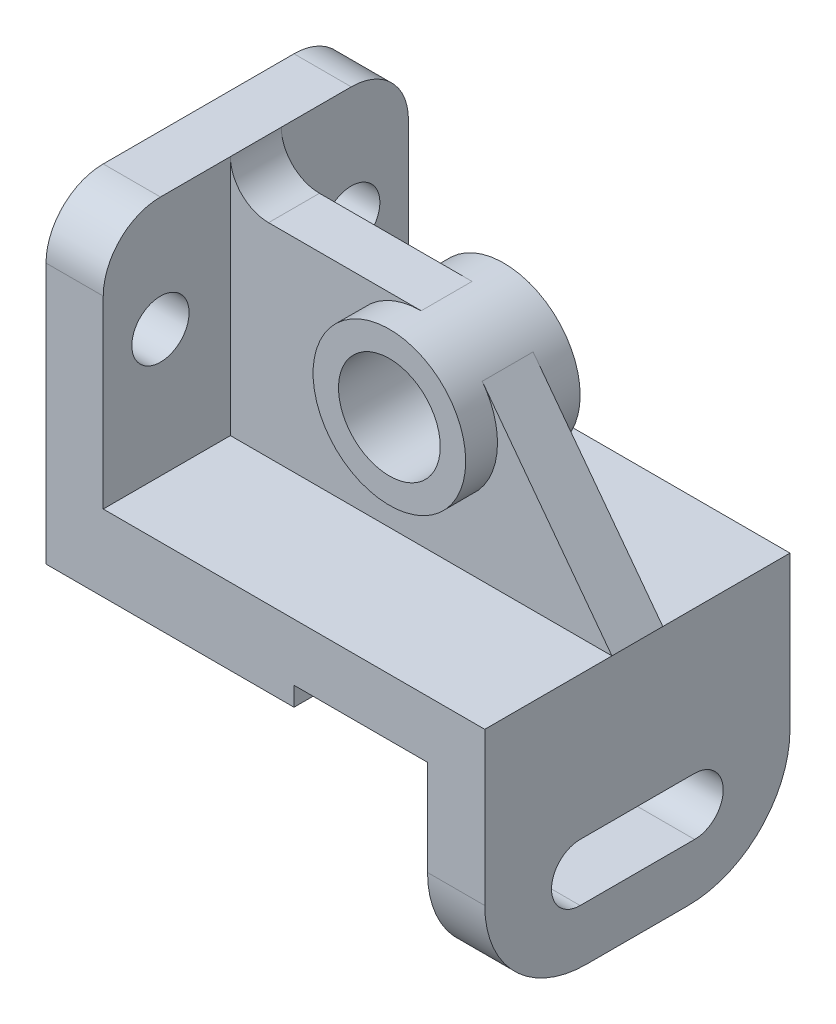
ISO-10303-21;
HEADER;
FILE_DESCRIPTION(('STEP AP214'),'2;1');
FILE_NAME('part.step','',(''),(''),'','','');
FILE_SCHEMA(('AUTOMOTIVE_DESIGN { 1 0 10303 214 1 1 1 1 }'));
ENDSEC;
DATA;
#1=APPLICATION_CONTEXT('core data for automotive mechanical design processes');
#2=APPLICATION_PROTOCOL_DEFINITION('international standard','automotive_design',2000,#1);
#3=PRODUCT_CONTEXT('',#1,'mechanical');
#4=PRODUCT('Part','Part','',(#3));
#5=PRODUCT_RELATED_PRODUCT_CATEGORY('part','',(#4));
#6=PRODUCT_DEFINITION_FORMATION('','',#4);
#7=PRODUCT_DEFINITION_CONTEXT('part definition',#1,'design');
#8=PRODUCT_DEFINITION('design','',#6,#7);
#9=PRODUCT_DEFINITION_SHAPE('','',#8);
#10=(LENGTH_UNIT() NAMED_UNIT(*) SI_UNIT(.MILLI.,.METRE.));
#11=(NAMED_UNIT(*) PLANE_ANGLE_UNIT() SI_UNIT($,.RADIAN.));
#12=(NAMED_UNIT(*) SI_UNIT($,.STERADIAN.) SOLID_ANGLE_UNIT());
#13=UNCERTAINTY_MEASURE_WITH_UNIT(LENGTH_MEASURE(1.E-05),#10,'distance_accuracy_value','');
#14=(GEOMETRIC_REPRESENTATION_CONTEXT(3) GLOBAL_UNCERTAINTY_ASSIGNED_CONTEXT((#13)) GLOBAL_UNIT_ASSIGNED_CONTEXT((#10,
#11,#12)) REPRESENTATION_CONTEXT('',''));
#15=CARTESIAN_POINT('',(0.,0.,0.));
#16=DIRECTION('',(0.,0.,1.));
#17=DIRECTION('',(1.,0.,0.));
#18=AXIS2_PLACEMENT_3D('',#15,#16,#17);
#19=CARTESIAN_POINT('',(69.,12.,-48.));
#20=DIRECTION('',(0.,1.,0.));
#21=DIRECTION('',(0.,0.,1.));
#22=AXIS2_PLACEMENT_3D('',#19,#20,#21);
#23=PLANE('',#22);
#24=DIRECTION('',(0.,0.,1.));
#25=VECTOR('',#24,1.);
#26=CARTESIAN_POINT('',(9.,12.,-48.));
#27=LINE('',#26,#25);
#28=CARTESIAN_POINT('',(9.,12.,-48.));
#29=VERTEX_POINT('',#28);
#30=CARTESIAN_POINT('',(9.,12.,-28.));
#31=VERTEX_POINT('',#30);
#32=EDGE_CURVE('E272',#29,#31,#27,.T.);
#33=ORIENTED_EDGE('',*,*,#32,.T.);
#34=DIRECTION('',(1.,0.,0.));
#35=VECTOR('',#34,1.);
#36=CARTESIAN_POINT('',(69.,12.,-28.));
#37=LINE('',#36,#35);
#38=CARTESIAN_POINT('',(69.,12.,-28.));
#39=VERTEX_POINT('',#38);
#40=EDGE_CURVE('E492',#31,#39,#37,.T.);
#41=ORIENTED_EDGE('',*,*,#40,.T.);
#42=DIRECTION('',(0.,0.,1.));
#43=VECTOR('',#42,1.);
#44=CARTESIAN_POINT('',(69.,12.,-48.));
#45=LINE('',#44,#43);
#46=CARTESIAN_POINT('',(69.,12.,-48.));
#47=VERTEX_POINT('',#46);
#48=EDGE_CURVE('E351',#47,#39,#45,.T.);
#49=ORIENTED_EDGE('',*,*,#48,.F.);
#50=DIRECTION('',(-1.,0.,0.));
#51=VECTOR('',#50,1.);
#52=CARTESIAN_POINT('',(69.,12.,-48.));
#53=LINE('',#52,#51);
#54=EDGE_CURVE('E331',#47,#29,#53,.T.);
#55=ORIENTED_EDGE('',*,*,#54,.T.);
#56=EDGE_LOOP('',(#33,#41,#49,#55));
#57=FACE_BOUND('',#56,.T.);
#58=ADVANCED_FACE('F44',(#57),#23,.T.);
#59=CARTESIAN_POINT('',(9.,0.,0.));
#60=DIRECTION('',(-1.,0.,0.));
#61=DIRECTION('',(0.,0.,1.));
#62=AXIS2_PLACEMENT_3D('',#59,#60,#61);
#63=PLANE('',#62);
#64=CARTESIAN_POINT('',(9.,32.,-39.));
#65=DIRECTION('',(-1.,0.,0.));
#66=DIRECTION('',(0.,0.,1.));
#67=AXIS2_PLACEMENT_3D('',#64,#65,#66);
#68=CIRCLE('',#67,4.5);
#69=CARTESIAN_POINT('',(9.,32.,-34.5));
#70=VERTEX_POINT('',#69);
#71=EDGE_CURVE('E286',#70,#70,#68,.T.);
#72=ORIENTED_EDGE('',*,*,#71,.T.);
#73=EDGE_LOOP('',(#72));
#74=FACE_BOUND('',#73,.T.);
#75=DIRECTION('',(0.,-1.,0.));
#76=VECTOR('',#75,1.);
#77=CARTESIAN_POINT('',(9.,50.,-48.));
#78=LINE('',#77,#76);
#79=CARTESIAN_POINT('',(9.,41.,-48.));
#80=VERTEX_POINT('',#79);
#81=EDGE_CURVE('E297',#80,#29,#78,.T.);
#82=ORIENTED_EDGE('',*,*,#81,.F.);
#83=CARTESIAN_POINT('',(9.,41.,-39.));
#84=DIRECTION('',(-1.,0.,0.));
#85=DIRECTION('',(0.,0.,1.));
#86=AXIS2_PLACEMENT_3D('',#83,#84,#85);
#87=CIRCLE('',#86,9.);
#88=CARTESIAN_POINT('',(9.,50.,-39.));
#89=VERTEX_POINT('',#88);
#90=EDGE_CURVE('E11',#80,#89,#87,.F.);
#91=ORIENTED_EDGE('',*,*,#90,.T.);
#92=DIRECTION('',(0.,0.,-1.));
#93=VECTOR('',#92,1.);
#94=CARTESIAN_POINT('',(9.,50.,0.));
#95=LINE('',#94,#93);
#96=CARTESIAN_POINT('',(9.,50.,-28.));
#97=VERTEX_POINT('',#96);
#98=EDGE_CURVE('E275',#97,#89,#95,.T.);
#99=ORIENTED_EDGE('',*,*,#98,.F.);
#100=DIRECTION('',(0.,-1.,0.));
#101=VECTOR('',#100,1.);
#102=CARTESIAN_POINT('',(9.,12.,-28.));
#103=LINE('',#102,#101);
#104=EDGE_CURVE('E479',#97,#31,#103,.T.);
#105=ORIENTED_EDGE('',*,*,#104,.T.);
#106=ORIENTED_EDGE('',*,*,#32,.F.);
#107=EDGE_LOOP('',(#82,#91,#99,#105,#106));
#108=FACE_BOUND('',#107,.T.);
#109=ADVANCED_FACE('F460',(#74,#108),#63,.F.);
#110=DIRECTION('',(1.,0.,0.));
#111=VECTOR('',#110,1.);
#112=CARTESIAN_POINT('',(69.,12.,-20.));
#113=LINE('',#112,#111);
#114=CARTESIAN_POINT('',(9.,12.,-20.));
#115=VERTEX_POINT('',#114);
#116=CARTESIAN_POINT('',(69.,12.,-20.));
#117=VERTEX_POINT('',#116);
#118=EDGE_CURVE('E475',#115,#117,#113,.T.);
#119=ORIENTED_EDGE('',*,*,#118,.F.);
#120=CARTESIAN_POINT('',(9.,12.,0.));
#121=VERTEX_POINT('',#120);
#122=EDGE_CURVE('E290',#115,#121,#27,.T.);
#123=ORIENTED_EDGE('',*,*,#122,.T.);
#124=DIRECTION('',(-1.,0.,0.));
#125=VECTOR('',#124,1.);
#126=CARTESIAN_POINT('',(69.,12.,0.));
#127=LINE('',#126,#125);
#128=CARTESIAN_POINT('',(69.,12.,0.));
#129=VERTEX_POINT('',#128);
#130=EDGE_CURVE('E271',#129,#121,#127,.T.);
#131=ORIENTED_EDGE('',*,*,#130,.F.);
#132=EDGE_CURVE('E356',#117,#129,#45,.T.);
#133=ORIENTED_EDGE('',*,*,#132,.F.);
#134=EDGE_LOOP('',(#119,#123,#131,#133));
#135=FACE_BOUND('',#134,.T.);
#136=ADVANCED_FACE('F458',(#135),#23,.T.);
#137=CARTESIAN_POINT('',(0.,12.,-48.));
#138=DIRECTION('',(-1.,0.,0.));
#139=DIRECTION('',(0.,0.,1.));
#140=AXIS2_PLACEMENT_3D('',#137,#138,#139);
#141=PLANE('',#140);
#142=DIRECTION('',(0.,-1.,0.));
#143=VECTOR('',#142,1.);
#144=CARTESIAN_POINT('',(0.,12.,0.));
#145=LINE('',#144,#143);
#146=CARTESIAN_POINT('',(0.,41.,0.));
#147=VERTEX_POINT('',#146);
#148=CARTESIAN_POINT('',(0.,0.,0.));
#149=VERTEX_POINT('',#148);
#150=EDGE_CURVE('E285',#147,#149,#145,.T.);
#151=ORIENTED_EDGE('',*,*,#150,.F.);
#152=CARTESIAN_POINT('',(0.,41.,-9.));
#153=DIRECTION('',(-1.,0.,0.));
#154=DIRECTION('',(0.,0.,1.));
#155=AXIS2_PLACEMENT_3D('',#152,#153,#154);
#156=CIRCLE('',#155,9.);
#157=CARTESIAN_POINT('',(0.,50.,-9.));
#158=VERTEX_POINT('',#157);
#159=EDGE_CURVE('E241',#147,#158,#156,.T.);
#160=ORIENTED_EDGE('',*,*,#159,.T.);
#161=DIRECTION('',(0.,0.,-1.));
#162=VECTOR('',#161,1.);
#163=CARTESIAN_POINT('',(0.,50.,0.));
#164=LINE('',#163,#162);
#165=CARTESIAN_POINT('',(0.,50.,-39.));
#166=VERTEX_POINT('',#165);
#167=EDGE_CURVE('E282',#158,#166,#164,.T.);
#168=ORIENTED_EDGE('',*,*,#167,.T.);
#169=CARTESIAN_POINT('',(0.,41.,-39.));
#170=DIRECTION('',(-1.,0.,0.));
#171=DIRECTION('',(0.,0.,1.));
#172=AXIS2_PLACEMENT_3D('',#169,#170,#171);
#173=CIRCLE('',#172,9.);
#174=CARTESIAN_POINT('',(0.,41.,-48.));
#175=VERTEX_POINT('',#174);
#176=EDGE_CURVE('E240',#166,#175,#173,.T.);
#177=ORIENTED_EDGE('',*,*,#176,.T.);
#178=DIRECTION('',(0.,-1.,0.));
#179=VECTOR('',#178,1.);
#180=CARTESIAN_POINT('',(0.,12.,-48.));
#181=LINE('',#180,#179);
#182=CARTESIAN_POINT('',(0.,0.,-48.));
#183=VERTEX_POINT('',#182);
#184=EDGE_CURVE('E318',#175,#183,#181,.T.);
#185=ORIENTED_EDGE('',*,*,#184,.T.);
#186=DIRECTION('',(0.,0.,1.));
#187=VECTOR('',#186,1.);
#188=CARTESIAN_POINT('',(0.,0.,-48.));
#189=LINE('',#188,#187);
#190=EDGE_CURVE('E339',#183,#149,#189,.T.);
#191=ORIENTED_EDGE('',*,*,#190,.T.);
#192=EDGE_LOOP('',(#151,#160,#168,#177,#185,#191));
#193=FACE_BOUND('',#192,.T.);
#194=CARTESIAN_POINT('',(0.,32.,-9.));
#195=DIRECTION('',(-1.,0.,0.));
#196=DIRECTION('',(0.,0.,1.));
#197=AXIS2_PLACEMENT_3D('',#194,#195,#196);
#198=CIRCLE('',#197,4.5);
#199=CARTESIAN_POINT('',(0.,32.,-4.50000000000001));
#200=VERTEX_POINT('',#199);
#201=EDGE_CURVE('E501',#200,#200,#198,.T.);
#202=ORIENTED_EDGE('',*,*,#201,.F.);
#203=EDGE_LOOP('',(#202));
#204=FACE_BOUND('',#203,.T.);
#205=CARTESIAN_POINT('',(0.,32.,-39.));
#206=DIRECTION('',(-1.,0.,0.));
#207=DIRECTION('',(0.,0.,1.));
#208=AXIS2_PLACEMENT_3D('',#205,#206,#207);
#209=CIRCLE('',#208,4.5);
#210=CARTESIAN_POINT('',(0.,32.,-34.5));
#211=VERTEX_POINT('',#210);
#212=EDGE_CURVE('E295',#211,#211,#209,.T.);
#213=ORIENTED_EDGE('',*,*,#212,.F.);
#214=EDGE_LOOP('',(#213));
#215=FACE_BOUND('',#214,.T.);
#216=ADVANCED_FACE('F276',(#193,#204,#215),#141,.T.);
#217=CARTESIAN_POINT('',(69.,-28.,-48.));
#218=DIRECTION('',(1.,0.,0.));
#219=DIRECTION('',(0.,0.,-1.));
#220=AXIS2_PLACEMENT_3D('',#217,#218,#219);
#221=PLANE('',#220);
#222=CARTESIAN_POINT('',(69.,-15.,-15.));
#223=DIRECTION('',(1.,0.,0.));
#224=DIRECTION('',(0.,0.,-1.));
#225=AXIS2_PLACEMENT_3D('',#222,#223,#224);
#226=CIRCLE('',#225,4.5);
#227=CARTESIAN_POINT('',(69.,-10.5,-15.));
#228=VERTEX_POINT('',#227);
#229=CARTESIAN_POINT('',(69.,-19.5,-15.));
#230=VERTEX_POINT('',#229);
#231=EDGE_CURVE('E300',#228,#230,#226,.T.);
#232=ORIENTED_EDGE('',*,*,#231,.F.);
#233=DIRECTION('',(0.,0.,1.));
#234=VECTOR('',#233,1.);
#235=CARTESIAN_POINT('',(69.,-10.5,-15.));
#236=LINE('',#235,#234);
#237=CARTESIAN_POINT('',(69.,-10.5,-33.));
#238=VERTEX_POINT('',#237);
#239=EDGE_CURVE('E308',#238,#228,#236,.T.);
#240=ORIENTED_EDGE('',*,*,#239,.F.);
#241=CARTESIAN_POINT('',(69.,-15.,-33.));
#242=DIRECTION('',(1.,0.,0.));
#243=DIRECTION('',(0.,0.,-1.));
#244=AXIS2_PLACEMENT_3D('',#241,#242,#243);
#245=CIRCLE('',#244,4.5);
#246=CARTESIAN_POINT('',(69.,-19.5,-33.));
#247=VERTEX_POINT('',#246);
#248=EDGE_CURVE('E301',#247,#238,#245,.T.);
#249=ORIENTED_EDGE('',*,*,#248,.F.);
#250=DIRECTION('',(0.,0.,-1.));
#251=VECTOR('',#250,1.);
#252=CARTESIAN_POINT('',(69.,-19.5,-15.));
#253=LINE('',#252,#251);
#254=EDGE_CURVE('E298',#230,#247,#253,.T.);
#255=ORIENTED_EDGE('',*,*,#254,.F.);
#256=EDGE_LOOP('',(#232,#240,#249,#255));
#257=FACE_BOUND('',#256,.T.);
#258=DIRECTION('',(0.,0.,1.));
#259=VECTOR('',#258,1.);
#260=CARTESIAN_POINT('',(69.,-28.,-48.));
#261=LINE('',#260,#259);
#262=CARTESIAN_POINT('',(69.,-28.,-32.));
#263=VERTEX_POINT('',#262);
#264=CARTESIAN_POINT('',(69.,-28.,-16.));
#265=VERTEX_POINT('',#264);
#266=EDGE_CURVE('E357',#263,#265,#261,.T.);
#267=ORIENTED_EDGE('',*,*,#266,.F.);
#268=CARTESIAN_POINT('',(69.,-12.,-32.));
#269=DIRECTION('',(1.,0.,0.));
#270=DIRECTION('',(0.,0.,-1.));
#271=AXIS2_PLACEMENT_3D('',#268,#269,#270);
#272=CIRCLE('',#271,16.);
#273=CARTESIAN_POINT('',(69.,-12.,-48.));
#274=VERTEX_POINT('',#273);
#275=EDGE_CURVE('E377',#263,#274,#272,.T.);
#276=ORIENTED_EDGE('',*,*,#275,.T.);
#277=DIRECTION('',(0.,1.,0.));
#278=VECTOR('',#277,1.);
#279=CARTESIAN_POINT('',(69.,-28.,-48.));
#280=LINE('',#279,#278);
#281=EDGE_CURVE('E335',#274,#47,#280,.T.);
#282=ORIENTED_EDGE('',*,*,#281,.T.);
#283=ORIENTED_EDGE('',*,*,#48,.T.);
#284=DIRECTION('',(0.,0.,-1.));
#285=VECTOR('',#284,1.);
#286=CARTESIAN_POINT('',(69.,12.,-20.));
#287=LINE('',#286,#285);
#288=EDGE_CURVE('E502',#117,#39,#287,.T.);
#289=ORIENTED_EDGE('',*,*,#288,.F.);
#290=ORIENTED_EDGE('',*,*,#132,.T.);
#291=DIRECTION('',(0.,1.,0.));
#292=VECTOR('',#291,1.);
#293=CARTESIAN_POINT('',(69.,-28.,0.));
#294=LINE('',#293,#292);
#295=CARTESIAN_POINT('',(69.,-12.,0.));
#296=VERTEX_POINT('',#295);
#297=EDGE_CURVE('E352',#296,#129,#294,.T.);
#298=ORIENTED_EDGE('',*,*,#297,.F.);
#299=CARTESIAN_POINT('',(69.,-12.,-16.));
#300=DIRECTION('',(1.,0.,0.));
#301=DIRECTION('',(0.,0.,-1.));
#302=AXIS2_PLACEMENT_3D('',#299,#300,#301);
#303=CIRCLE('',#302,16.);
#304=EDGE_CURVE('E380',#296,#265,#303,.T.);
#305=ORIENTED_EDGE('',*,*,#304,.T.);
#306=EDGE_LOOP('',(#267,#276,#282,#283,#289,#290,#298,#305));
#307=FACE_BOUND('',#306,.T.);
#308=ADVANCED_FACE('F417',(#257,#307),#221,.T.);
#309=CARTESIAN_POINT('',(60.,-28.,-48.));
#310=DIRECTION('',(0.,-1.,0.));
#311=DIRECTION('',(0.,0.,-1.));
#312=AXIS2_PLACEMENT_3D('',#309,#310,#311);
#313=PLANE('',#312);
#314=DIRECTION('',(0.,0.,1.));
#315=VECTOR('',#314,1.);
#316=CARTESIAN_POINT('',(60.,-28.,-48.));
#317=LINE('',#316,#315);
#318=CARTESIAN_POINT('',(60.,-28.,-32.));
#319=VERTEX_POINT('',#318);
#320=CARTESIAN_POINT('',(60.,-28.,-16.));
#321=VERTEX_POINT('',#320);
#322=EDGE_CURVE('E362',#319,#321,#317,.T.);
#323=ORIENTED_EDGE('',*,*,#322,.F.);
#324=DIRECTION('',(1.,0.,0.));
#325=VECTOR('',#324,1.);
#326=CARTESIAN_POINT('',(69.,-28.,-32.));
#327=LINE('',#326,#325);
#328=EDGE_CURVE('E372',#319,#263,#327,.T.);
#329=ORIENTED_EDGE('',*,*,#328,.T.);
#330=ORIENTED_EDGE('',*,*,#266,.T.);
#331=DIRECTION('',(1.,0.,0.));
#332=VECTOR('',#331,1.);
#333=CARTESIAN_POINT('',(60.,-28.,-16.));
#334=LINE('',#333,#332);
#335=EDGE_CURVE('E360',#265,#321,#334,.F.);
#336=ORIENTED_EDGE('',*,*,#335,.T.);
#337=EDGE_LOOP('',(#323,#329,#330,#336));
#338=FACE_BOUND('',#337,.T.);
#339=ADVANCED_FACE('F419',(#338),#313,.T.);
#340=CARTESIAN_POINT('',(60.,0.,-48.));
#341=DIRECTION('',(-1.,0.,0.));
#342=DIRECTION('',(0.,0.,1.));
#343=AXIS2_PLACEMENT_3D('',#340,#341,#342);
#344=PLANE('',#343);
#345=CARTESIAN_POINT('',(60.,-15.,-15.));
#346=DIRECTION('',(-1.,0.,0.));
#347=DIRECTION('',(0.,0.,1.));
#348=AXIS2_PLACEMENT_3D('',#345,#346,#347);
#349=CIRCLE('',#348,4.5);
#350=CARTESIAN_POINT('',(60.,-19.5,-15.));
#351=VERTEX_POINT('',#350);
#352=CARTESIAN_POINT('',(60.,-10.5,-15.));
#353=VERTEX_POINT('',#352);
#354=EDGE_CURVE('E232',#351,#353,#349,.T.);
#355=ORIENTED_EDGE('',*,*,#354,.F.);
#356=DIRECTION('',(0.,0.,1.));
#357=VECTOR('',#356,1.);
#358=CARTESIAN_POINT('',(60.,-19.5,-48.));
#359=LINE('',#358,#357);
#360=CARTESIAN_POINT('',(60.,-19.5,-33.));
#361=VERTEX_POINT('',#360);
#362=EDGE_CURVE('E388',#361,#351,#359,.T.);
#363=ORIENTED_EDGE('',*,*,#362,.F.);
#364=CARTESIAN_POINT('',(60.,-15.,-33.));
#365=DIRECTION('',(-1.,0.,0.));
#366=DIRECTION('',(0.,0.,1.));
#367=AXIS2_PLACEMENT_3D('',#364,#365,#366);
#368=CIRCLE('',#367,4.5);
#369=CARTESIAN_POINT('',(60.,-10.5,-33.));
#370=VERTEX_POINT('',#369);
#371=EDGE_CURVE('E394',#370,#361,#368,.T.);
#372=ORIENTED_EDGE('',*,*,#371,.F.);
#373=DIRECTION('',(0.,0.,-1.));
#374=VECTOR('',#373,1.);
#375=CARTESIAN_POINT('',(60.,-10.5,-48.));
#376=LINE('',#375,#374);
#377=EDGE_CURVE('E239',#353,#370,#376,.T.);
#378=ORIENTED_EDGE('',*,*,#377,.F.);
#379=EDGE_LOOP('',(#355,#363,#372,#378));
#380=FACE_BOUND('',#379,.T.);
#381=DIRECTION('',(0.,-1.,0.));
#382=VECTOR('',#381,1.);
#383=CARTESIAN_POINT('',(60.,3.,-48.));
#384=LINE('',#383,#382);
#385=CARTESIAN_POINT('',(60.,3.,-48.));
#386=VERTEX_POINT('',#385);
#387=CARTESIAN_POINT('',(60.,-12.,-48.));
#388=VERTEX_POINT('',#387);
#389=EDGE_CURVE('E328',#386,#388,#384,.T.);
#390=ORIENTED_EDGE('',*,*,#389,.T.);
#391=CARTESIAN_POINT('',(60.,-12.,-32.));
#392=DIRECTION('',(-1.,0.,0.));
#393=DIRECTION('',(0.,0.,1.));
#394=AXIS2_PLACEMENT_3D('',#391,#392,#393);
#395=CIRCLE('',#394,16.);
#396=EDGE_CURVE('E384',#388,#319,#395,.T.);
#397=ORIENTED_EDGE('',*,*,#396,.T.);
#398=ORIENTED_EDGE('',*,*,#322,.T.);
#399=CARTESIAN_POINT('',(60.,-12.,-16.));
#400=DIRECTION('',(-1.,0.,0.));
#401=DIRECTION('',(0.,0.,1.));
#402=AXIS2_PLACEMENT_3D('',#399,#400,#401);
#403=CIRCLE('',#402,16.);
#404=CARTESIAN_POINT('',(60.,-12.,0.));
#405=VERTEX_POINT('',#404);
#406=EDGE_CURVE('E382',#321,#405,#403,.T.);
#407=ORIENTED_EDGE('',*,*,#406,.T.);
#408=DIRECTION('',(0.,-1.,0.));
#409=VECTOR('',#408,1.);
#410=CARTESIAN_POINT('',(60.,0.,0.));
#411=LINE('',#410,#409);
#412=CARTESIAN_POINT('',(60.,3.,0.));
#413=VERTEX_POINT('',#412);
#414=EDGE_CURVE('E346',#413,#405,#411,.T.);
#415=ORIENTED_EDGE('',*,*,#414,.F.);
#416=DIRECTION('',(0.,0.,1.));
#417=VECTOR('',#416,1.);
#418=CARTESIAN_POINT('',(60.,3.,-48.));
#419=LINE('',#418,#417);
#420=EDGE_CURVE('E364',#386,#413,#419,.T.);
#421=ORIENTED_EDGE('',*,*,#420,.F.);
#422=EDGE_LOOP('',(#390,#397,#398,#407,#415,#421));
#423=FACE_BOUND('',#422,.T.);
#424=ADVANCED_FACE('F409',(#380,#423),#344,.T.);
#425=CARTESIAN_POINT('',(39.,3.,-48.));
#426=DIRECTION('',(0.,-1.,0.));
#427=DIRECTION('',(0.,0.,-1.));
#428=AXIS2_PLACEMENT_3D('',#425,#426,#427);
#429=PLANE('',#428);
#430=DIRECTION('',(1.,0.,0.));
#431=VECTOR('',#430,1.);
#432=CARTESIAN_POINT('',(39.,3.,0.));
#433=LINE('',#432,#431);
#434=CARTESIAN_POINT('',(39.,3.,0.));
#435=VERTEX_POINT('',#434);
#436=EDGE_CURVE('E344',#435,#413,#433,.T.);
#437=ORIENTED_EDGE('',*,*,#436,.F.);
#438=DIRECTION('',(0.,0.,1.));
#439=VECTOR('',#438,1.);
#440=CARTESIAN_POINT('',(39.,3.,-48.));
#441=LINE('',#440,#439);
#442=CARTESIAN_POINT('',(39.,3.,-48.));
#443=VERTEX_POINT('',#442);
#444=EDGE_CURVE('E366',#443,#435,#441,.T.);
#445=ORIENTED_EDGE('',*,*,#444,.F.);
#446=DIRECTION('',(1.,0.,0.));
#447=VECTOR('',#446,1.);
#448=CARTESIAN_POINT('',(39.,3.,-48.));
#449=LINE('',#448,#447);
#450=EDGE_CURVE('E326',#443,#386,#449,.T.);
#451=ORIENTED_EDGE('',*,*,#450,.T.);
#452=ORIENTED_EDGE('',*,*,#420,.T.);
#453=EDGE_LOOP('',(#437,#445,#451,#452));
#454=FACE_BOUND('',#453,.T.);
#455=ADVANCED_FACE('F436',(#454),#429,.T.);
#456=CARTESIAN_POINT('',(39.,0.,-48.));
#457=DIRECTION('',(1.,0.,0.));
#458=DIRECTION('',(0.,0.,-1.));
#459=AXIS2_PLACEMENT_3D('',#456,#457,#458);
#460=PLANE('',#459);
#461=DIRECTION('',(0.,1.,0.));
#462=VECTOR('',#461,1.);
#463=CARTESIAN_POINT('',(39.,0.,0.));
#464=LINE('',#463,#462);
#465=CARTESIAN_POINT('',(39.,0.,0.));
#466=VERTEX_POINT('',#465);
#467=EDGE_CURVE('E345',#466,#435,#464,.T.);
#468=ORIENTED_EDGE('',*,*,#467,.F.);
#469=DIRECTION('',(0.,0.,1.));
#470=VECTOR('',#469,1.);
#471=CARTESIAN_POINT('',(39.,0.,-48.));
#472=LINE('',#471,#470);
#473=CARTESIAN_POINT('',(39.,0.,-48.));
#474=VERTEX_POINT('',#473);
#475=EDGE_CURVE('E367',#474,#466,#472,.T.);
#476=ORIENTED_EDGE('',*,*,#475,.F.);
#477=DIRECTION('',(0.,1.,0.));
#478=VECTOR('',#477,1.);
#479=CARTESIAN_POINT('',(39.,0.,-48.));
#480=LINE('',#479,#478);
#481=EDGE_CURVE('E323',#474,#443,#480,.T.);
#482=ORIENTED_EDGE('',*,*,#481,.T.);
#483=ORIENTED_EDGE('',*,*,#444,.T.);
#484=EDGE_LOOP('',(#468,#476,#482,#483));
#485=FACE_BOUND('',#484,.T.);
#486=ADVANCED_FACE('F520',(#485),#460,.T.);
#487=CARTESIAN_POINT('',(0.,0.,-48.));
#488=DIRECTION('',(0.,-1.,0.));
#489=DIRECTION('',(0.,0.,-1.));
#490=AXIS2_PLACEMENT_3D('',#487,#488,#489);
#491=PLANE('',#490);
#492=DIRECTION('',(1.,0.,0.));
#493=VECTOR('',#492,1.);
#494=CARTESIAN_POINT('',(0.,0.,0.));
#495=LINE('',#494,#493);
#496=EDGE_CURVE('E336',#149,#466,#495,.T.);
#497=ORIENTED_EDGE('',*,*,#496,.F.);
#498=ORIENTED_EDGE('',*,*,#190,.F.);
#499=DIRECTION('',(1.,0.,0.));
#500=VECTOR('',#499,1.);
#501=CARTESIAN_POINT('',(0.,0.,-48.));
#502=LINE('',#501,#500);
#503=EDGE_CURVE('E319',#183,#474,#502,.T.);
#504=ORIENTED_EDGE('',*,*,#503,.T.);
#505=ORIENTED_EDGE('',*,*,#475,.T.);
#506=EDGE_LOOP('',(#497,#498,#504,#505));
#507=FACE_BOUND('',#506,.T.);
#508=ADVANCED_FACE('F517',(#507),#491,.T.);
#509=CARTESIAN_POINT('',(0.,0.,-48.));
#510=DIRECTION('',(0.,0.,1.));
#511=DIRECTION('',(1.,0.,0.));
#512=AXIS2_PLACEMENT_3D('',#509,#510,#511);
#513=PLANE('',#512);
#514=ORIENTED_EDGE('',*,*,#184,.F.);
#515=DIRECTION('',(-1.,0.,0.));
#516=VECTOR('',#515,1.);
#517=CARTESIAN_POINT('',(9.,41.,-48.));
#518=LINE('',#517,#516);
#519=EDGE_CURVE('E52',#175,#80,#518,.F.);
#520=ORIENTED_EDGE('',*,*,#519,.T.);
#521=ORIENTED_EDGE('',*,*,#81,.T.);
#522=ORIENTED_EDGE('',*,*,#54,.F.);
#523=ORIENTED_EDGE('',*,*,#281,.F.);
#524=DIRECTION('',(1.,0.,0.));
#525=VECTOR('',#524,1.);
#526=CARTESIAN_POINT('',(60.,-12.,-48.));
#527=LINE('',#526,#525);
#528=EDGE_CURVE('E381',#274,#388,#527,.F.);
#529=ORIENTED_EDGE('',*,*,#528,.T.);
#530=ORIENTED_EDGE('',*,*,#389,.F.);
#531=ORIENTED_EDGE('',*,*,#450,.F.);
#532=ORIENTED_EDGE('',*,*,#481,.F.);
#533=ORIENTED_EDGE('',*,*,#503,.F.);
#534=EDGE_LOOP('',(#514,#520,#521,#522,#523,#529,#530,#531,#532,#533));
#535=FACE_BOUND('',#534,.T.);
#536=ADVANCED_FACE('F439',(#535),#513,.F.);
#537=CARTESIAN_POINT('',(0.,0.,0.));
#538=DIRECTION('',(0.,0.,1.));
#539=DIRECTION('',(1.,0.,0.));
#540=AXIS2_PLACEMENT_3D('',#537,#538,#539);
#541=PLANE('',#540);
#542=DIRECTION('',(0.,1.,0.));
#543=VECTOR('',#542,1.);
#544=CARTESIAN_POINT('',(9.,12.,0.));
#545=LINE('',#544,#543);
#546=CARTESIAN_POINT('',(9.,41.,0.));
#547=VERTEX_POINT('',#546);
#548=EDGE_CURVE('E259',#121,#547,#545,.T.);
#549=ORIENTED_EDGE('',*,*,#548,.T.);
#550=DIRECTION('',(-1.,0.,0.));
#551=VECTOR('',#550,1.);
#552=CARTESIAN_POINT('',(0.,41.,0.));
#553=LINE('',#552,#551);
#554=EDGE_CURVE('E231',#547,#147,#553,.T.);
#555=ORIENTED_EDGE('',*,*,#554,.T.);
#556=ORIENTED_EDGE('',*,*,#150,.T.);
#557=ORIENTED_EDGE('',*,*,#496,.T.);
#558=ORIENTED_EDGE('',*,*,#467,.T.);
#559=ORIENTED_EDGE('',*,*,#436,.T.);
#560=ORIENTED_EDGE('',*,*,#414,.T.);
#561=DIRECTION('',(1.,0.,0.));
#562=VECTOR('',#561,1.);
#563=CARTESIAN_POINT('',(0.,-12.,0.));
#564=LINE('',#563,#562);
#565=EDGE_CURVE('E390',#405,#296,#564,.T.);
#566=ORIENTED_EDGE('',*,*,#565,.T.);
#567=ORIENTED_EDGE('',*,*,#297,.T.);
#568=ORIENTED_EDGE('',*,*,#130,.T.);
#569=EDGE_LOOP('',(#549,#555,#556,#557,#558,#559,#560,#566,#567,#568));
#570=FACE_BOUND('',#569,.T.);
#571=ADVANCED_FACE('F270',(#570),#541,.T.);
#572=CARTESIAN_POINT('',(60.,-12.,-32.));
#573=DIRECTION('',(-1.,0.,0.));
#574=DIRECTION('',(0.,0.,1.));
#575=AXIS2_PLACEMENT_3D('',#572,#573,#574);
#576=CYLINDRICAL_SURFACE('',#575,16.);
#577=ORIENTED_EDGE('',*,*,#396,.F.);
#578=ORIENTED_EDGE('',*,*,#528,.F.);
#579=ORIENTED_EDGE('',*,*,#275,.F.);
#580=ORIENTED_EDGE('',*,*,#328,.F.);
#581=EDGE_LOOP('',(#577,#578,#579,#580));
#582=FACE_BOUND('',#581,.T.);
#583=ADVANCED_FACE('F443',(#582),#576,.T.);
#584=CARTESIAN_POINT('',(0.,-12.,-16.));
#585=DIRECTION('',(1.,0.,0.));
#586=DIRECTION('',(0.,0.,-1.));
#587=AXIS2_PLACEMENT_3D('',#584,#585,#586);
#588=CYLINDRICAL_SURFACE('',#587,16.);
#589=ORIENTED_EDGE('',*,*,#406,.F.);
#590=ORIENTED_EDGE('',*,*,#335,.F.);
#591=ORIENTED_EDGE('',*,*,#304,.F.);
#592=ORIENTED_EDGE('',*,*,#565,.F.);
#593=EDGE_LOOP('',(#589,#590,#591,#592));
#594=FACE_BOUND('',#593,.T.);
#595=ADVANCED_FACE('F431',(#594),#588,.T.);
#596=CARTESIAN_POINT('',(21.,-15.,-15.));
#597=DIRECTION('',(1.,0.,0.));
#598=DIRECTION('',(0.,0.,-1.));
#599=AXIS2_PLACEMENT_3D('',#596,#597,#598);
#600=CYLINDRICAL_SURFACE('',#599,4.5);
#601=ORIENTED_EDGE('',*,*,#354,.T.);
#602=DIRECTION('',(1.,0.,0.));
#603=VECTOR('',#602,1.);
#604=CARTESIAN_POINT('',(21.,-10.5,-15.));
#605=LINE('',#604,#603);
#606=EDGE_CURVE('E309',#353,#228,#605,.T.);
#607=ORIENTED_EDGE('',*,*,#606,.T.);
#608=ORIENTED_EDGE('',*,*,#231,.T.);
#609=DIRECTION('',(1.,0.,0.));
#610=VECTOR('',#609,1.);
#611=CARTESIAN_POINT('',(21.,-19.5,-15.));
#612=LINE('',#611,#610);
#613=EDGE_CURVE('E310',#351,#230,#612,.T.);
#614=ORIENTED_EDGE('',*,*,#613,.F.);
#615=EDGE_LOOP('',(#601,#607,#608,#614));
#616=FACE_BOUND('',#615,.T.);
#617=ADVANCED_FACE('F412',(#616),#600,.F.);
#618=CARTESIAN_POINT('',(21.,-10.5,-15.));
#619=DIRECTION('',(0.,1.,0.));
#620=DIRECTION('',(0.,0.,1.));
#621=AXIS2_PLACEMENT_3D('',#618,#619,#620);
#622=PLANE('',#621);
#623=ORIENTED_EDGE('',*,*,#377,.T.);
#624=DIRECTION('',(1.,0.,0.));
#625=VECTOR('',#624,1.);
#626=CARTESIAN_POINT('',(21.,-10.5,-33.));
#627=LINE('',#626,#625);
#628=EDGE_CURVE('E315',#370,#238,#627,.T.);
#629=ORIENTED_EDGE('',*,*,#628,.T.);
#630=ORIENTED_EDGE('',*,*,#239,.T.);
#631=ORIENTED_EDGE('',*,*,#606,.F.);
#632=EDGE_LOOP('',(#623,#629,#630,#631));
#633=FACE_BOUND('',#632,.T.);
#634=ADVANCED_FACE('F396',(#633),#622,.F.);
#635=CARTESIAN_POINT('',(21.,-15.,-33.));
#636=DIRECTION('',(1.,0.,0.));
#637=DIRECTION('',(0.,0.,-1.));
#638=AXIS2_PLACEMENT_3D('',#635,#636,#637);
#639=CYLINDRICAL_SURFACE('',#638,4.5);
#640=ORIENTED_EDGE('',*,*,#371,.T.);
#641=DIRECTION('',(1.,0.,0.));
#642=VECTOR('',#641,1.);
#643=CARTESIAN_POINT('',(21.,-19.5,-33.));
#644=LINE('',#643,#642);
#645=EDGE_CURVE('E314',#361,#247,#644,.T.);
#646=ORIENTED_EDGE('',*,*,#645,.T.);
#647=ORIENTED_EDGE('',*,*,#248,.T.);
#648=ORIENTED_EDGE('',*,*,#628,.F.);
#649=EDGE_LOOP('',(#640,#646,#647,#648));
#650=FACE_BOUND('',#649,.T.);
#651=ADVANCED_FACE('F401',(#650),#639,.F.);
#652=CARTESIAN_POINT('',(21.,-19.5,-15.));
#653=DIRECTION('',(0.,-1.,0.));
#654=DIRECTION('',(0.,0.,-1.));
#655=AXIS2_PLACEMENT_3D('',#652,#653,#654);
#656=PLANE('',#655);
#657=ORIENTED_EDGE('',*,*,#362,.T.);
#658=ORIENTED_EDGE('',*,*,#613,.T.);
#659=ORIENTED_EDGE('',*,*,#254,.T.);
#660=ORIENTED_EDGE('',*,*,#645,.F.);
#661=EDGE_LOOP('',(#657,#658,#659,#660));
#662=FACE_BOUND('',#661,.T.);
#663=ADVANCED_FACE('F413',(#662),#656,.F.);
#664=CARTESIAN_POINT('',(9.,50.,0.));
#665=DIRECTION('',(0.,1.,0.));
#666=DIRECTION('',(0.,0.,1.));
#667=AXIS2_PLACEMENT_3D('',#664,#665,#666);
#668=PLANE('',#667);
#669=ORIENTED_EDGE('',*,*,#167,.F.);
#670=DIRECTION('',(-1.,0.,0.));
#671=VECTOR('',#670,1.);
#672=CARTESIAN_POINT('',(9.,50.,-9.));
#673=LINE('',#672,#671);
#674=CARTESIAN_POINT('',(9.,50.,-9.));
#675=VERTEX_POINT('',#674);
#676=EDGE_CURVE('E247',#158,#675,#673,.F.);
#677=ORIENTED_EDGE('',*,*,#676,.T.);
#678=CARTESIAN_POINT('',(9.,50.,-20.));
#679=VERTEX_POINT('',#678);
#680=EDGE_CURVE('E265',#675,#679,#95,.T.);
#681=ORIENTED_EDGE('',*,*,#680,.T.);
#682=DIRECTION('',(0.,0.,-1.));
#683=VECTOR('',#682,1.);
#684=CARTESIAN_POINT('',(9.,50.,-20.));
#685=LINE('',#684,#683);
#686=EDGE_CURVE('E490',#679,#97,#685,.T.);
#687=ORIENTED_EDGE('',*,*,#686,.T.);
#688=ORIENTED_EDGE('',*,*,#98,.T.);
#689=DIRECTION('',(-1.,0.,0.));
#690=VECTOR('',#689,1.);
#691=CARTESIAN_POINT('',(0.,50.,-39.));
#692=LINE('',#691,#690);
#693=EDGE_CURVE('E248',#89,#166,#692,.T.);
#694=ORIENTED_EDGE('',*,*,#693,.T.);
#695=EDGE_LOOP('',(#669,#677,#681,#687,#688,#694));
#696=FACE_BOUND('',#695,.T.);
#697=ADVANCED_FACE('F283',(#696),#668,.T.);
#698=CARTESIAN_POINT('',(9.,32.,-9.));
#699=DIRECTION('',(-1.,0.,0.));
#700=DIRECTION('',(0.,0.,1.));
#701=AXIS2_PLACEMENT_3D('',#698,#699,#700);
#702=CIRCLE('',#701,4.5);
#703=CARTESIAN_POINT('',(9.,32.,-4.50000000000001));
#704=VERTEX_POINT('',#703);
#705=EDGE_CURVE('E503',#704,#704,#702,.T.);
#706=ORIENTED_EDGE('',*,*,#705,.T.);
#707=EDGE_LOOP('',(#706));
#708=FACE_BOUND('',#707,.T.);
#709=ORIENTED_EDGE('',*,*,#680,.F.);
#710=CARTESIAN_POINT('',(9.,41.,-9.));
#711=DIRECTION('',(-1.,0.,0.));
#712=DIRECTION('',(0.,0.,1.));
#713=AXIS2_PLACEMENT_3D('',#710,#711,#712);
#714=CIRCLE('',#713,9.);
#715=EDGE_CURVE('E253',#675,#547,#714,.F.);
#716=ORIENTED_EDGE('',*,*,#715,.T.);
#717=ORIENTED_EDGE('',*,*,#548,.F.);
#718=ORIENTED_EDGE('',*,*,#122,.F.);
#719=DIRECTION('',(0.,-1.,0.));
#720=VECTOR('',#719,1.);
#721=CARTESIAN_POINT('',(9.,12.,-20.));
#722=LINE('',#721,#720);
#723=EDGE_CURVE('E481',#679,#115,#722,.T.);
#724=ORIENTED_EDGE('',*,*,#723,.F.);
#725=EDGE_LOOP('',(#709,#716,#717,#718,#724));
#726=FACE_BOUND('',#725,.T.);
#727=ADVANCED_FACE('F260',(#708,#726),#63,.F.);
#728=CARTESIAN_POINT('',(9.,32.,-39.));
#729=DIRECTION('',(-1.,0.,0.));
#730=DIRECTION('',(0.,0.,1.));
#731=AXIS2_PLACEMENT_3D('',#728,#729,#730);
#732=CYLINDRICAL_SURFACE('',#731,4.5);
#733=ORIENTED_EDGE('',*,*,#71,.F.);
#734=EDGE_LOOP('',(#733));
#735=FACE_BOUND('',#734,.T.);
#736=ORIENTED_EDGE('',*,*,#212,.T.);
#737=EDGE_LOOP('',(#736));
#738=FACE_BOUND('',#737,.T.);
#739=ADVANCED_FACE('F644',(#735,#738),#732,.F.);
#740=CARTESIAN_POINT('',(9.,32.,-9.));
#741=DIRECTION('',(-1.,0.,0.));
#742=DIRECTION('',(0.,0.,1.));
#743=AXIS2_PLACEMENT_3D('',#740,#741,#742);
#744=CYLINDRICAL_SURFACE('',#743,4.5);
#745=ORIENTED_EDGE('',*,*,#705,.F.);
#746=EDGE_LOOP('',(#745));
#747=FACE_BOUND('',#746,.T.);
#748=ORIENTED_EDGE('',*,*,#201,.T.);
#749=EDGE_LOOP('',(#748));
#750=FACE_BOUND('',#749,.T.);
#751=ADVANCED_FACE('F701',(#747,#750),#744,.F.);
#752=CARTESIAN_POINT('',(69.,12.,-20.));
#753=DIRECTION('',(-0.8,-0.6,0.));
#754=DIRECTION('',(0.6,-0.8,0.));
#755=AXIS2_PLACEMENT_3D('',#752,#753,#754);
#756=PLANE('',#755);
#757=DIRECTION('',(-0.6,0.8,0.));
#758=VECTOR('',#757,1.);
#759=CARTESIAN_POINT('',(69.,12.,-28.));
#760=LINE('',#759,#758);
#761=CARTESIAN_POINT('',(48.6,39.2,-28.));
#762=VERTEX_POINT('',#761);
#763=EDGE_CURVE('E220',#39,#762,#760,.T.);
#764=ORIENTED_EDGE('',*,*,#763,.T.);
#765=DIRECTION('',(0.,0.,-1.));
#766=VECTOR('',#765,1.);
#767=CARTESIAN_POINT('',(48.6,39.2,-20.));
#768=LINE('',#767,#766);
#769=CARTESIAN_POINT('',(48.6,39.2,-20.));
#770=VERTEX_POINT('',#769);
#771=EDGE_CURVE('E227',#770,#762,#768,.T.);
#772=ORIENTED_EDGE('',*,*,#771,.F.);
#773=DIRECTION('',(-0.6,0.8,0.));
#774=VECTOR('',#773,1.);
#775=CARTESIAN_POINT('',(69.,12.,-20.));
#776=LINE('',#775,#774);
#777=EDGE_CURVE('E476',#117,#770,#776,.T.);
#778=ORIENTED_EDGE('',*,*,#777,.F.);
#779=ORIENTED_EDGE('',*,*,#288,.T.);
#780=EDGE_LOOP('',(#764,#772,#778,#779));
#781=FACE_BOUND('',#780,.T.);
#782=ADVANCED_FACE('F691',(#781),#756,.F.);
#783=CARTESIAN_POINT('',(39.,44.,-20.));
#784=DIRECTION('',(0.,-1.,0.));
#785=DIRECTION('',(0.,0.,-1.));
#786=AXIS2_PLACEMENT_3D('',#783,#784,#785);
#787=PLANE('',#786);
#788=DIRECTION('',(-1.,0.,0.));
#789=VECTOR('',#788,1.);
#790=CARTESIAN_POINT('',(39.,44.,-28.));
#791=LINE('',#790,#789);
#792=CARTESIAN_POINT('',(39.,44.,-28.));
#793=VERTEX_POINT('',#792);
#794=CARTESIAN_POINT('',(15.,44.,-28.));
#795=VERTEX_POINT('',#794);
#796=EDGE_CURVE('E204',#793,#795,#791,.T.);
#797=ORIENTED_EDGE('',*,*,#796,.T.);
#798=DIRECTION('',(0.,0.,-1.));
#799=VECTOR('',#798,1.);
#800=CARTESIAN_POINT('',(15.,44.,-20.));
#801=LINE('',#800,#799);
#802=CARTESIAN_POINT('',(15.,44.,-20.));
#803=VERTEX_POINT('',#802);
#804=EDGE_CURVE('E229',#803,#795,#801,.T.);
#805=ORIENTED_EDGE('',*,*,#804,.F.);
#806=DIRECTION('',(-1.,0.,0.));
#807=VECTOR('',#806,1.);
#808=CARTESIAN_POINT('',(39.,44.,-20.));
#809=LINE('',#808,#807);
#810=CARTESIAN_POINT('',(39.,44.,-20.));
#811=VERTEX_POINT('',#810);
#812=EDGE_CURVE('E224',#811,#803,#809,.T.);
#813=ORIENTED_EDGE('',*,*,#812,.F.);
#814=DIRECTION('',(0.,0.,-1.));
#815=VECTOR('',#814,1.);
#816=CARTESIAN_POINT('',(39.,44.,-20.));
#817=LINE('',#816,#815);
#818=EDGE_CURVE('E222',#811,#793,#817,.T.);
#819=ORIENTED_EDGE('',*,*,#818,.T.);
#820=EDGE_LOOP('',(#797,#805,#813,#819));
#821=FACE_BOUND('',#820,.T.);
#822=ADVANCED_FACE('F225',(#821),#787,.F.);
#823=CARTESIAN_POINT('',(15.,50.,-20.));
#824=DIRECTION('',(0.,0.,-1.));
#825=DIRECTION('',(-1.,0.,0.));
#826=AXIS2_PLACEMENT_3D('',#823,#824,#825);
#827=CYLINDRICAL_SURFACE('',#826,6.00000000000001);
#828=CARTESIAN_POINT('',(15.,50.,-28.));
#829=DIRECTION('',(0.,0.,-1.));
#830=DIRECTION('',(1.,0.,0.));
#831=AXIS2_PLACEMENT_3D('',#828,#829,#830);
#832=CIRCLE('',#831,6.00000000000001);
#833=EDGE_CURVE('E213',#795,#97,#832,.T.);
#834=ORIENTED_EDGE('',*,*,#833,.T.);
#835=ORIENTED_EDGE('',*,*,#686,.F.);
#836=CARTESIAN_POINT('',(15.,50.,-20.));
#837=DIRECTION('',(0.,0.,-1.));
#838=DIRECTION('',(1.,0.,0.));
#839=AXIS2_PLACEMENT_3D('',#836,#837,#838);
#840=CIRCLE('',#839,6.00000000000001);
#841=EDGE_CURVE('E484',#803,#679,#840,.T.);
#842=ORIENTED_EDGE('',*,*,#841,.F.);
#843=ORIENTED_EDGE('',*,*,#804,.T.);
#844=EDGE_LOOP('',(#834,#835,#842,#843));
#845=FACE_BOUND('',#844,.T.);
#846=ADVANCED_FACE('F680',(#845),#827,.F.);
#847=CARTESIAN_POINT('',(15.,50.,-20.));
#848=DIRECTION('',(0.,0.,1.));
#849=DIRECTION('',(1.,0.,0.));
#850=AXIS2_PLACEMENT_3D('',#847,#848,#849);
#851=PLANE('',#850);
#852=ORIENTED_EDGE('',*,*,#777,.T.);
#853=CARTESIAN_POINT('',(39.,32.,-20.));
#854=DIRECTION('',(0.,0.,1.));
#855=DIRECTION('',(1.,0.,0.));
#856=AXIS2_PLACEMENT_3D('',#853,#854,#855);
#857=CIRCLE('',#856,12.);
#858=EDGE_CURVE('E494',#770,#811,#857,.F.);
#859=ORIENTED_EDGE('',*,*,#858,.T.);
#860=ORIENTED_EDGE('',*,*,#812,.T.);
#861=ORIENTED_EDGE('',*,*,#841,.T.);
#862=ORIENTED_EDGE('',*,*,#723,.T.);
#863=ORIENTED_EDGE('',*,*,#118,.T.);
#864=EDGE_LOOP('',(#852,#859,#860,#861,#862,#863));
#865=FACE_BOUND('',#864,.T.);
#866=ADVANCED_FACE('F483',(#865),#851,.T.);
#867=CARTESIAN_POINT('',(15.,50.,-28.));
#868=DIRECTION('',(0.,0.,1.));
#869=DIRECTION('',(1.,0.,0.));
#870=AXIS2_PLACEMENT_3D('',#867,#868,#869);
#871=PLANE('',#870);
#872=CARTESIAN_POINT('',(39.,32.,-28.));
#873=DIRECTION('',(0.,0.,1.));
#874=DIRECTION('',(1.,0.,0.));
#875=AXIS2_PLACEMENT_3D('',#872,#873,#874);
#876=CIRCLE('',#875,12.);
#877=EDGE_CURVE('E207',#762,#793,#876,.F.);
#878=ORIENTED_EDGE('',*,*,#877,.F.);
#879=ORIENTED_EDGE('',*,*,#763,.F.);
#880=ORIENTED_EDGE('',*,*,#40,.F.);
#881=ORIENTED_EDGE('',*,*,#104,.F.);
#882=ORIENTED_EDGE('',*,*,#833,.F.);
#883=ORIENTED_EDGE('',*,*,#796,.F.);
#884=EDGE_LOOP('',(#878,#879,#880,#881,#882,#883));
#885=FACE_BOUND('',#884,.T.);
#886=ADVANCED_FACE('F206',(#885),#871,.F.);
#887=CARTESIAN_POINT('',(39.,32.,-15.));
#888=DIRECTION('',(0.,0.,-1.));
#889=DIRECTION('',(-1.,0.,0.));
#890=AXIS2_PLACEMENT_3D('',#887,#888,#889);
#891=CYLINDRICAL_SURFACE('',#890,8.);
#892=CARTESIAN_POINT('',(39.,32.,-33.));
#893=DIRECTION('',(0.,0.,1.));
#894=DIRECTION('',(1.,0.,0.));
#895=AXIS2_PLACEMENT_3D('',#892,#893,#894);
#896=CIRCLE('',#895,8.);
#897=CARTESIAN_POINT('',(47.,32.,-33.));
#898=VERTEX_POINT('',#897);
#899=EDGE_CURVE('E812',#898,#898,#896,.T.);
#900=ORIENTED_EDGE('',*,*,#899,.F.);
#901=EDGE_LOOP('',(#900));
#902=FACE_BOUND('',#901,.T.);
#903=CARTESIAN_POINT('',(39.,32.,-15.));
#904=DIRECTION('',(0.,0.,1.));
#905=DIRECTION('',(1.,0.,0.));
#906=AXIS2_PLACEMENT_3D('',#903,#904,#905);
#907=CIRCLE('',#906,8.);
#908=CARTESIAN_POINT('',(47.,32.,-15.));
#909=VERTEX_POINT('',#908);
#910=EDGE_CURVE('E811',#909,#909,#907,.T.);
#911=ORIENTED_EDGE('',*,*,#910,.T.);
#912=EDGE_LOOP('',(#911));
#913=FACE_BOUND('',#912,.T.);
#914=ADVANCED_FACE('F666',(#902,#913),#891,.F.);
#915=CARTESIAN_POINT('',(39.,32.,-15.));
#916=DIRECTION('',(0.,0.,1.));
#917=DIRECTION('',(1.,0.,0.));
#918=AXIS2_PLACEMENT_3D('',#915,#916,#917);
#919=PLANE('',#918);
#920=CARTESIAN_POINT('',(39.,32.,-15.));
#921=DIRECTION('',(0.,0.,1.));
#922=DIRECTION('',(1.,0.,0.));
#923=AXIS2_PLACEMENT_3D('',#920,#921,#922);
#924=CIRCLE('',#923,12.);
#925=CARTESIAN_POINT('',(51.,32.,-15.));
#926=VERTEX_POINT('',#925);
#927=EDGE_CURVE('E810',#926,#926,#924,.T.);
#928=ORIENTED_EDGE('',*,*,#927,.T.);
#929=EDGE_LOOP('',(#928));
#930=FACE_BOUND('',#929,.T.);
#931=ORIENTED_EDGE('',*,*,#910,.F.);
#932=EDGE_LOOP('',(#931));
#933=FACE_BOUND('',#932,.T.);
#934=ADVANCED_FACE('F716',(#930,#933),#919,.T.);
#935=CARTESIAN_POINT('',(39.,32.,-33.));
#936=DIRECTION('',(0.,0.,1.));
#937=DIRECTION('',(1.,0.,0.));
#938=AXIS2_PLACEMENT_3D('',#935,#936,#937);
#939=PLANE('',#938);
#940=CARTESIAN_POINT('',(39.,32.,-33.));
#941=DIRECTION('',(0.,0.,1.));
#942=DIRECTION('',(1.,0.,0.));
#943=AXIS2_PLACEMENT_3D('',#940,#941,#942);
#944=CIRCLE('',#943,12.);
#945=CARTESIAN_POINT('',(51.,32.,-33.));
#946=VERTEX_POINT('',#945);
#947=EDGE_CURVE('E806',#946,#946,#944,.T.);
#948=ORIENTED_EDGE('',*,*,#947,.F.);
#949=EDGE_LOOP('',(#948));
#950=FACE_BOUND('',#949,.T.);
#951=ORIENTED_EDGE('',*,*,#899,.T.);
#952=EDGE_LOOP('',(#951));
#953=FACE_BOUND('',#952,.T.);
#954=ADVANCED_FACE('F709',(#950,#953),#939,.F.);
#955=CARTESIAN_POINT('',(39.,32.,-15.));
#956=DIRECTION('',(0.,0.,-1.));
#957=DIRECTION('',(-1.,0.,0.));
#958=AXIS2_PLACEMENT_3D('',#955,#956,#957);
#959=CYLINDRICAL_SURFACE('',#958,12.);
#960=ORIENTED_EDGE('',*,*,#858,.F.);
#961=ORIENTED_EDGE('',*,*,#771,.T.);
#962=ORIENTED_EDGE('',*,*,#877,.T.);
#963=ORIENTED_EDGE('',*,*,#818,.F.);
#964=EDGE_LOOP('',(#960,#961,#962,#963));
#965=FACE_BOUND('',#964,.T.);
#966=ORIENTED_EDGE('',*,*,#927,.F.);
#967=EDGE_LOOP('',(#966));
#968=FACE_BOUND('',#967,.T.);
#969=ORIENTED_EDGE('',*,*,#947,.T.);
#970=EDGE_LOOP('',(#969));
#971=FACE_BOUND('',#970,.T.);
#972=ADVANCED_FACE('F228',(#965,#968,#971),#959,.T.);
#973=CARTESIAN_POINT('',(0.,41.,-9.));
#974=DIRECTION('',(-1.,0.,0.));
#975=DIRECTION('',(0.,0.,1.));
#976=AXIS2_PLACEMENT_3D('',#973,#974,#975);
#977=CYLINDRICAL_SURFACE('',#976,9.);
#978=ORIENTED_EDGE('',*,*,#715,.F.);
#979=ORIENTED_EDGE('',*,*,#676,.F.);
#980=ORIENTED_EDGE('',*,*,#159,.F.);
#981=ORIENTED_EDGE('',*,*,#554,.F.);
#982=EDGE_LOOP('',(#978,#979,#980,#981));
#983=FACE_BOUND('',#982,.T.);
#984=ADVANCED_FACE('F274',(#983),#977,.T.);
#985=CARTESIAN_POINT('',(9.,41.,-39.));
#986=DIRECTION('',(1.,0.,0.));
#987=DIRECTION('',(0.,0.,-1.));
#988=AXIS2_PLACEMENT_3D('',#985,#986,#987);
#989=CYLINDRICAL_SURFACE('',#988,9.);
#990=ORIENTED_EDGE('',*,*,#90,.F.);
#991=ORIENTED_EDGE('',*,*,#519,.F.);
#992=ORIENTED_EDGE('',*,*,#176,.F.);
#993=ORIENTED_EDGE('',*,*,#693,.F.);
#994=EDGE_LOOP('',(#990,#991,#992,#993));
#995=FACE_BOUND('',#994,.T.);
#996=ADVANCED_FACE('F50',(#995),#989,.T.);
#997=CLOSED_SHELL('',(#58,#109,#136,#216,#308,#339,#424,#455,#486,#508,#536,#571,#583,#595,#617,
#634,#651,#663,#697,#727,#739,#751,#782,#822,#846,#866,#886,#914,#934,#954,#972,#984,#996));
#998=MANIFOLD_SOLID_BREP('B2',#997);
#999=ADVANCED_BREP_SHAPE_REPRESENTATION('',(#18,#998),#14);
#1000=SHAPE_DEFINITION_REPRESENTATION(#9,#999);
ENDSEC;
END-ISO-10303-21;
